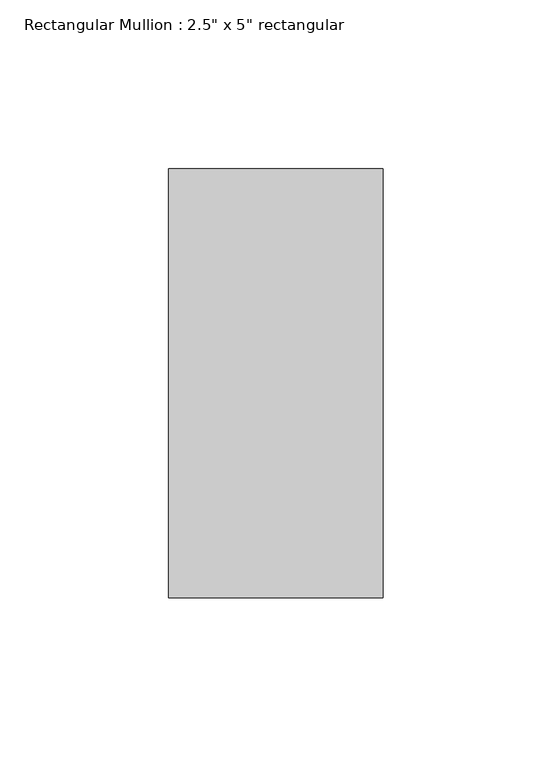
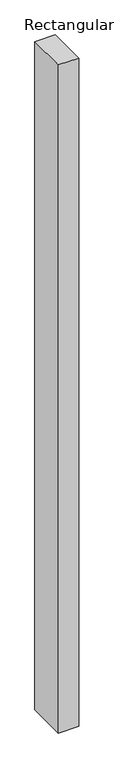
"""IFC4 building model written with IfcOpenShell, lengths in millimetres: member geometry."""

from ifc_helpers import new_model, si_unit, frame, origin, place, context, project, spatial, polyline, outline, extrude, source, transform, mapped, element, save


def member_e3d2676c(model_context):
    return source(origin(), model_context, "Body", "SweptSolid", [
        extrude(outline(polyline([(0.0, 63.5), (0.0, -63.5), (-63.5, -63.5), (-63.5, 63.5), (0.0, 63.5)])), frame((0.0, 0.0, -2208.0093941), z_axis=(0.0, 0.0, 1.0), x_axis=(1.0, 0.0, 0.0)), (0.0, 0.0, 1.0), 2208.0093941),
    ])


if __name__ == "__main__":
    model = new_model("IFC4")
    model_context = context("Model", 3, world=origin())
    ifc_project = project(units=[si_unit("LENGTHUNIT", "METRE", prefix="MILLI")], contexts=[model_context])
    site = spatial("IfcSite", under=ifc_project)
    building = spatial("IfcBuilding", under=site)
    placement = place(None, origin())
    member_shape = member_e3d2676c(model_context)
    element("IfcMember", 1, ObjectType="Rectangular Mullion : 2.5\" x 5\" rectangular", at=placement, inside=building, context=model_context, shape_type="MappedRepresentation", body=[
        mapped(member_shape, transform((0.0, 0.0, 0.0), x_axis=(1.0, 0.0, 0.0), y_axis=(0.0, 1.0, 0.0), z_axis=(0.0, 0.0, 1.0))),
    ])
    save(model, "model.ifc")

# Revit data of these elements
# Type "Rectangular Mullion : 2.5\" x 5\" rectangular"
#   built-in parameter 1007304 = 0.416667 (stored number, unit not read)
#   built-in parameter 1007301 = 0.104167 (stored number, unit not read)
#   built-in parameter 1007300 = 0.104167 (stored number, unit not read)
